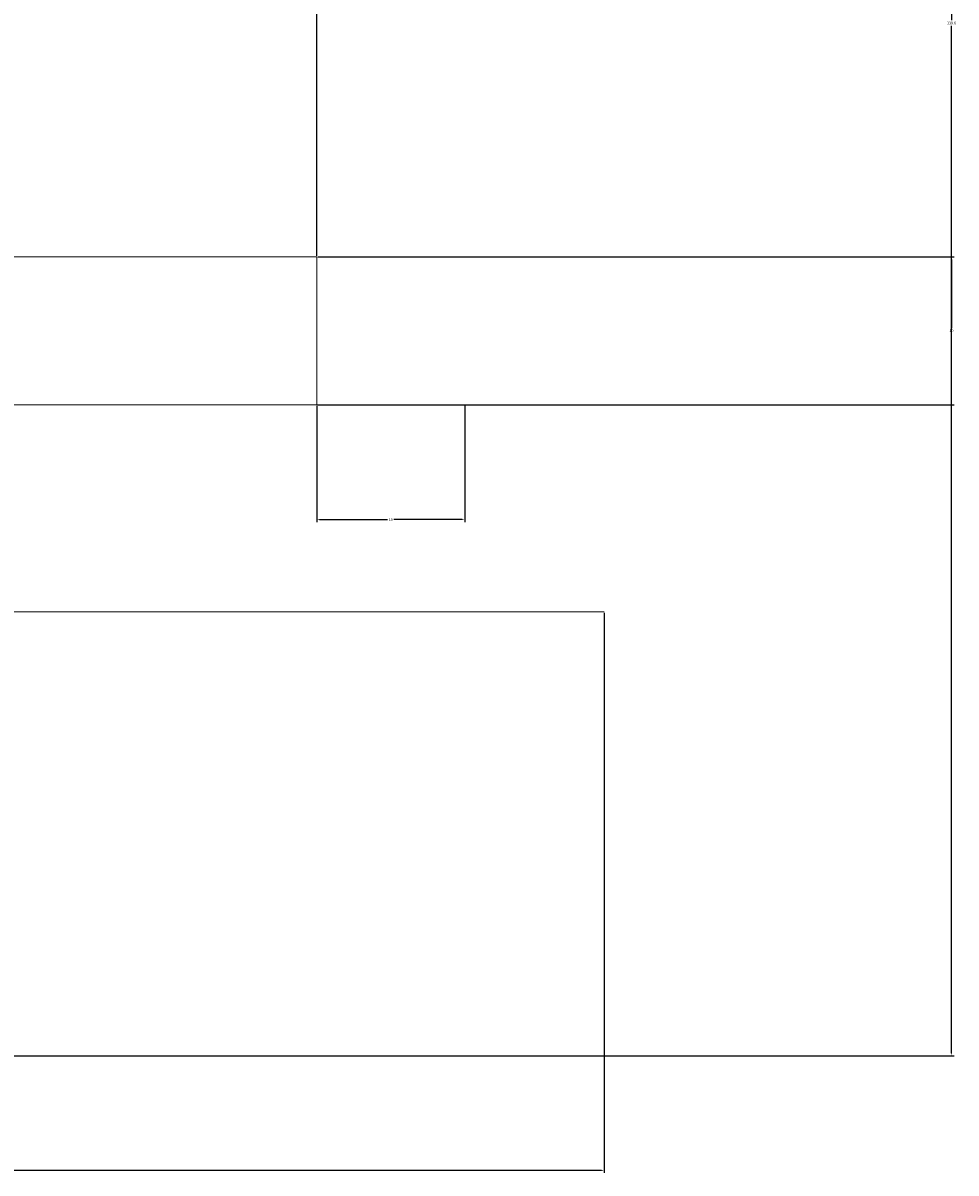
# Model space of a CAD drawing. Units: millimetres. Extents: x 118 to 244, y 285 to 440.
# Tile 3 of 4: x 181 to 244, y 285 to 362. Entities that reach past the tile are written whole.
import ezdxf

# ---------------------------------------------------------------- set-up
doc = ezdxf.new("R2010")
doc.units = ezdxf.units.MM
doc.layers.add('M-CONS', color=8, linetype='Continuous', lineweight=13)
doc.layers.add('M-DIMS', color=2, linetype='Continuous', lineweight=18)
doc.styles.get("Standard").update_dxf_attribs({"font": 'arial.ttf'})
doc.dimstyles.get("Standard").update_dxf_attribs({"dimtxt": 0.18, "dimasz": 0.18, "dimexe": 0.18, "dimexo": 0.0625, "dimgap": 0.09, "dimtad": 0, "dimtih": 1, "dimtoh": 1, "dimdec": 4, "dimzin": 0, "dimdsep": 46, "dimtxsty": 'Standard', "dimcen": 0.09, "dimadec": 0, "dimazin": 0, "dimtfac": 1, "dimtdec": 4, "dimtofl": 0, "dimtmove": 0, "dimatfit": 3, "dimfxl": 1, "dimtolj": 1, "dimtzin": 0, "dimarcsym": 0})

# ---------------------------------------------------------------- blocks, each defined once
blk = doc.blocks.new('*D1')
at = {"layer": 'Defpoints', "color": 0, "transparency": 16777216}
for p in [(219.95, 322.437), (125.524, 292.437), (219.95, 284.687)]:
    blk.add_point(p, dxfattribs=at)
at = {"layer": 'M-DIMS', "color": 0, "lineweight": -2, "transparency": 16777216}
for p, q in [((219.95, 322.374), (219.95, 284.507)), ((125.524, 292.374), (125.524, 284.507)), ((125.704, 284.687), (172.343, 284.687)), ((219.77, 284.687), (173.131, 284.687))]:
    blk.add_line(p, q, dxfattribs=at)
at = {"layer": 'M-DIMS', "color": 0, "transparency": 16777216}
for points in [[(125.704, 284.717), (125.704, 284.657), (125.524, 284.687)], [(219.77, 284.717), (219.77, 284.657), (219.95, 284.687)]]:
    blk.add_solid(points, dxfattribs=at)
at = {"layer": 'M-DIMS', "color": 0, "transparency": 16777216, "insert": (172.737, 284.687), "char_height": 0.18, "attachment_point": 5}
blk.add_mtext('\\A1;94.43', dxfattribs=at)
blk = doc.blocks.new('*D3')
at = {"layer": 'Defpoints', "color": 0, "transparency": 16777216}
for p in [(200.524, 439.795), (125.524, 346.437), (200.524, 346.437)]:
    blk.add_point(p, dxfattribs=at)
at = {"layer": 'M-DIMS', "color": 0, "lineweight": -2, "transparency": 16777216}
for p, q in [((125.524, 346.499), (125.524, 439.975)), ((200.524, 346.499), (200.524, 439.975)), ((125.704, 439.795), (162.805, 439.795)), ((200.344, 439.795), (163.243, 439.795))]:
    blk.add_line(p, q, dxfattribs=at)
at = {"layer": 'M-DIMS', "color": 0, "transparency": 16777216}
for points in [[(125.704, 439.825), (125.704, 439.765), (125.524, 439.795)], [(200.344, 439.825), (200.344, 439.765), (200.524, 439.795)]]:
    blk.add_solid(points, dxfattribs=at)
at = {"layer": 'M-DIMS', "color": 0, "transparency": 16777216, "insert": (163.024, 439.795), "char_height": 0.18, "attachment_point": 5}
blk.add_mtext('\\A1;75', dxfattribs=at)
blk = doc.blocks.new('*D4')
at = {"layer": 'Defpoints', "color": 0, "transparency": 16777216}
for p in [(200.524, 346.437), (200.524, 336.437), (243.427, 336.437)]:
    blk.add_point(p, dxfattribs=at)
at = {"layer": 'M-DIMS', "color": 0, "lineweight": -2, "transparency": 16777216}
for p, q in [((200.587, 346.437), (243.607, 346.437)), ((243.427, 346.257), (243.427, 341.619)), ((243.427, 336.617), (243.427, 341.255)), ((200.587, 336.437), (243.607, 336.437))]:
    blk.add_line(p, q, dxfattribs=at)
at = {"layer": 'M-DIMS', "color": 0, "transparency": 16777216}
for points in [[(243.397, 346.257), (243.457, 346.257), (243.427, 346.437)], [(243.397, 336.617), (243.457, 336.617), (243.427, 336.437)]]:
    blk.add_solid(points, dxfattribs=at)
at = {"layer": 'M-DIMS', "color": 0, "transparency": 16777216, "insert": (243.427, 341.437), "char_height": 0.18, "attachment_point": 5}
blk.add_mtext('\\A1;10', dxfattribs=at)
blk = doc.blocks.new('*D5')
at = {"layer": 'Defpoints', "color": 0, "transparency": 16777216}
for p in [(200.524, 336.437), (210.524, 336.437), (200.524, 328.687)]:
    blk.add_point(p, dxfattribs=at)
at = {"layer": 'M-DIMS', "color": 0, "lineweight": -2, "transparency": 16777216}
for p, q in [((200.524, 336.374), (200.524, 328.507)), ((210.524, 336.374), (210.524, 328.507)), ((200.704, 328.687), (205.314, 328.687)), ((210.344, 328.687), (205.734, 328.687))]:
    blk.add_line(p, q, dxfattribs=at)
at = {"layer": 'M-DIMS', "color": 0, "transparency": 16777216}
for points in [[(200.704, 328.717), (200.704, 328.657), (200.524, 328.687)], [(210.344, 328.717), (210.344, 328.657), (210.524, 328.687)]]:
    blk.add_solid(points, dxfattribs=at)
at = {"layer": 'M-DIMS', "color": 0, "transparency": 16777216, "insert": (205.524, 328.687), "char_height": 0.18, "attachment_point": 5}
blk.add_mtext('\\A1;10', dxfattribs=at)
blk = doc.blocks.new('*D9')
at = {"layer": 'Defpoints', "color": 0, "transparency": 16777216}
for p in [(235.677, 439.795), (235.677, 432.045), (125.524, 346.437)]:
    blk.add_point(p, dxfattribs=at)
at = {"layer": 'M-DIMS', "color": 0, "lineweight": -2, "transparency": 16777216}
for p, q in [((125.524, 346.499), (125.524, 439.975)), ((235.677, 432.107), (235.677, 439.975)), ((125.704, 439.795), (180.145, 439.795)), ((235.497, 439.795), (181.056, 439.795))]:
    blk.add_line(p, q, dxfattribs=at)
at = {"layer": 'M-DIMS', "color": 0, "transparency": 16777216}
for points in [[(125.704, 439.825), (125.704, 439.765), (125.524, 439.795)], [(235.497, 439.825), (235.497, 439.765), (235.677, 439.795)]]:
    blk.add_solid(points, dxfattribs=at)
at = {"layer": 'M-DIMS', "color": 0, "transparency": 16777216, "insert": (180.6, 439.795), "char_height": 0.18, "attachment_point": 5}
blk.add_mtext('\\A1;110.15', dxfattribs=at)
blk = doc.blocks.new('*D10')
at = {"layer": 'Defpoints', "color": 0, "transparency": 16777216}
for p in [(235.677, 432.045), (243.427, 432.045), (125.524, 292.437)]:
    blk.add_point(p, dxfattribs=at)
at = {"layer": 'M-DIMS', "color": 0, "lineweight": -2, "transparency": 16777216}
for p, q in [((235.739, 432.045), (243.607, 432.045)), ((243.427, 431.865), (243.427, 362.423)), ((243.427, 292.617), (243.427, 362.059)), ((125.587, 292.437), (243.607, 292.437))]:
    blk.add_line(p, q, dxfattribs=at)
at = {"layer": 'M-DIMS', "color": 0, "transparency": 16777216}
for points in [[(243.397, 431.865), (243.457, 431.865), (243.427, 432.045)], [(243.397, 292.617), (243.457, 292.617), (243.427, 292.437)]]:
    blk.add_solid(points, dxfattribs=at)
at = {"layer": 'M-DIMS', "color": 0, "transparency": 16777216, "insert": (243.427, 362.241), "char_height": 0.18, "attachment_point": 5}
blk.add_mtext('\\A1;139.6', dxfattribs=at)

msp = doc.modelspace()

# ---------------------------------------------------------------- linework, layer by layer
at = {"layer": 'M-CONS'}
for p, q in [((200.5241, 336.4369), (200.5241, 346.4369)), ((200.5241, 336.4369, 157.5697), (200.5241, 346.4369, 157.5697)), ((150.5241, 336.4369, 20), (210.5241, 336.4369, 20))]:
    msp.add_line(p, q, dxfattribs=at)
at = {"layer": 'M-CONS', "elevation": 10}
msp.add_lwpolyline([(125.5241, 336.4369), (155.5241, 336.4369), (200.5241, 336.4369), (200.5241, 346.4369), (125.5241, 346.4369)], close=True, dxfattribs=at)
at = {"layer": 'M-CONS', "extrusion": (0, 1, 0)}
msp.add_rational_spline([(150.0206, 322.4369, 167.5697), (172.4909, 322.4369, 167.5697), (194.9611, 322.4369, 167.5697), (219.9611, 322.4369, 167.5697), (219.9611, 322.4369, 142.5697)], [1, 1, 1, 0.707106781187, 1], degree=2, knots=[0, 0, 0, 1, 1, 2.5707963, 2.5707963, 2.5707963], dxfattribs=at)

# ---------------------------------------------------------------- dimensions: what is measured, and where the dimension line sits
at = {"layer": 'M-DIMS'}
for base, p1, p2, override, picture, middle in [((200.5241, 439.7945), (125.5241, 346.4369), (200.5241, 346.4369), {"dimdec": 0, "dimlfac": 1, "dimrnd": 0, "dimzin": 0, "dimdsep": 46, "dimlunit": 2}, '*D3', (163.0241, 439.7945)), ((235.6768, 439.7945), (125.5241, 346.4369), (235.6768, 432.0445), {"dimdec": 2, "dimlfac": 1, "dimrnd": 0, "dimzin": 0, "dimdsep": 46, "dimlunit": 2}, '*D9', (180.6005, 439.7945)), ((219.9501, 284.6869), (125.5241, 292.4369), (219.9501, 322.4369), {"dimdec": 2, "dimlfac": 1, "dimrnd": 0, "dimzin": 0, "dimdsep": 46, "dimlunit": 2}, '*D1', (172.7371, 284.6869))]:
    dim = msp.add_linear_dim(base=base, p1=p1, p2=p2, dimstyle='Standard', override=override, dxfattribs=at)
    dim.commit()
    dim.dimension.update_dxf_attribs({"geometry": picture, "text_midpoint": middle})
for base, p1, p2, angle, override, picture, middle in [((243.4268, 432.0445), (125.5241, 292.4369), (235.6768, 432.0445), 90, {"dimdec": 1, "dimlfac": 1, "dimrnd": 0, "dimzin": 0, "dimdsep": 46, "dimlunit": 2}, '*D10', (243.4268, 362.2407)), ((243.4268, 336.4369), (200.5241, 346.4369), (200.5241, 336.4369), 90, {"dimdec": 0, "dimlfac": 1, "dimrnd": 0, "dimzin": 0, "dimdsep": 46, "dimlunit": 2}, '*D4', (243.4268, 341.4369)), ((200.5241, 328.6869), (210.5241, 336.4369), (200.5241, 336.4369), 180, {"dimdec": 0, "dimlfac": 1, "dimrnd": 0, "dimzin": 0, "dimdsep": 46, "dimlunit": 2}, '*D5', (205.5241, 328.6869))]:
    dim = msp.add_linear_dim(base=base, p1=p1, p2=p2, angle=angle, dimstyle='Standard', override=override, dxfattribs=at)
    dim.commit()
    dim.dimension.update_dxf_attribs({"geometry": picture, "text_midpoint": middle})

doc.saveas('drawing.dxf')
